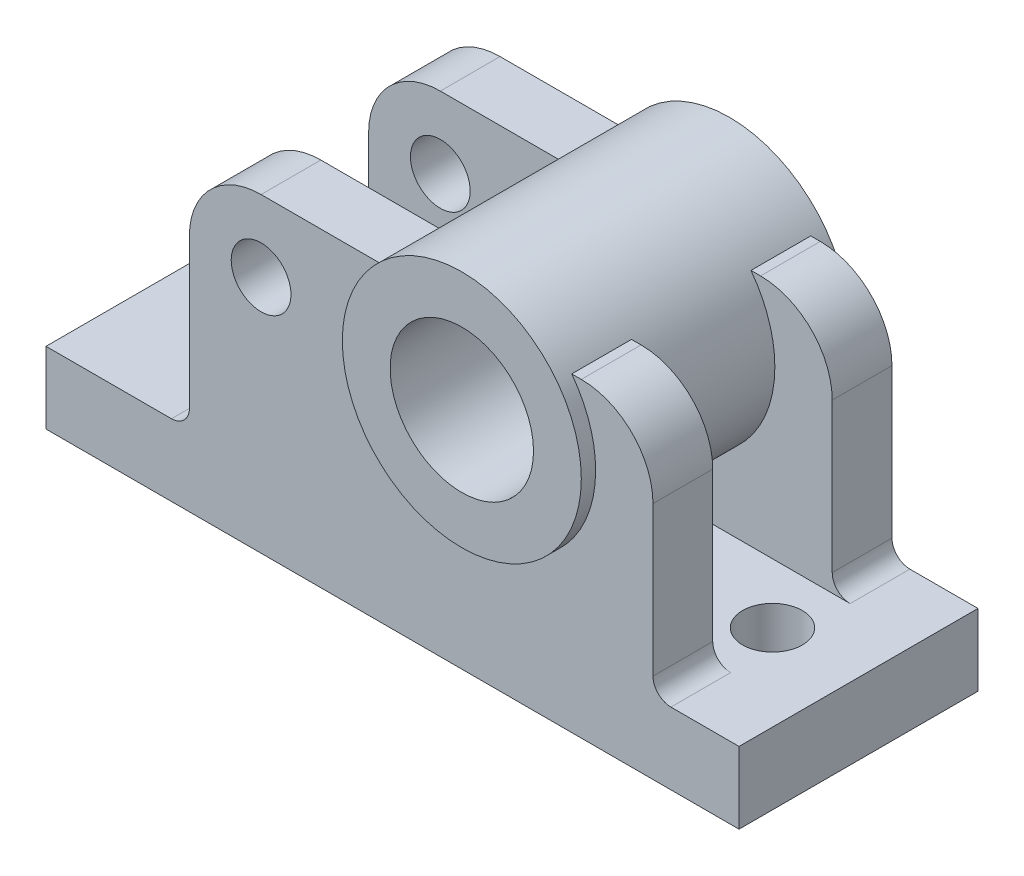
ISO-10303-21;
HEADER;
FILE_DESCRIPTION(('STEP AP214'),'2;1');
FILE_NAME('part.step','',(''),(''),'','','');
FILE_SCHEMA(('AUTOMOTIVE_DESIGN { 1 0 10303 214 1 1 1 1 }'));
ENDSEC;
DATA;
#1=APPLICATION_CONTEXT('core data for automotive mechanical design processes');
#2=APPLICATION_PROTOCOL_DEFINITION('international standard','automotive_design',2000,#1);
#3=PRODUCT_CONTEXT('',#1,'mechanical');
#4=PRODUCT('Part','Part','',(#3));
#5=PRODUCT_RELATED_PRODUCT_CATEGORY('part','',(#4));
#6=PRODUCT_DEFINITION_FORMATION('','',#4);
#7=PRODUCT_DEFINITION_CONTEXT('part definition',#1,'design');
#8=PRODUCT_DEFINITION('design','',#6,#7);
#9=PRODUCT_DEFINITION_SHAPE('','',#8);
#10=(LENGTH_UNIT() NAMED_UNIT(*) SI_UNIT(.MILLI.,.METRE.));
#11=(NAMED_UNIT(*) PLANE_ANGLE_UNIT() SI_UNIT($,.RADIAN.));
#12=(NAMED_UNIT(*) SI_UNIT($,.STERADIAN.) SOLID_ANGLE_UNIT());
#13=UNCERTAINTY_MEASURE_WITH_UNIT(LENGTH_MEASURE(1.E-05),#10,'distance_accuracy_value','');
#14=(GEOMETRIC_REPRESENTATION_CONTEXT(3) GLOBAL_UNCERTAINTY_ASSIGNED_CONTEXT((#13)) GLOBAL_UNIT_ASSIGNED_CONTEXT((#10,
#11,#12)) REPRESENTATION_CONTEXT('',''));
#15=CARTESIAN_POINT('',(0.,0.,0.));
#16=DIRECTION('',(0.,0.,1.));
#17=DIRECTION('',(1.,0.,0.));
#18=AXIS2_PLACEMENT_3D('',#15,#16,#17);
#19=CARTESIAN_POINT('',(110.,30.,50.));
#20=DIRECTION('',(0.,-1.,0.));
#21=DIRECTION('',(0.,0.,-1.));
#22=AXIS2_PLACEMENT_3D('',#19,#20,#21);
#23=PLANE('',#22);
#24=CARTESIAN_POINT('',(-144.,30.,0.));
#25=DIRECTION('',(0.,-1.,0.));
#26=DIRECTION('',(0.,0.,-1.));
#27=AXIS2_PLACEMENT_3D('',#24,#25,#26);
#28=CIRCLE('',#27,12.5);
#29=CARTESIAN_POINT('',(-144.,30.,-12.5));
#30=VERTEX_POINT('',#29);
#31=EDGE_CURVE('E249',#30,#30,#28,.T.);
#32=ORIENTED_EDGE('',*,*,#31,.T.);
#33=EDGE_LOOP('',(#32));
#34=FACE_BOUND('',#33,.T.);
#35=CARTESIAN_POINT('',(74.,30.,0.));
#36=DIRECTION('',(0.,-1.,0.));
#37=DIRECTION('',(0.,0.,-1.));
#38=AXIS2_PLACEMENT_3D('',#35,#36,#37);
#39=CIRCLE('',#38,12.5);
#40=CARTESIAN_POINT('',(74.,30.,-12.5));
#41=VERTEX_POINT('',#40);
#42=EDGE_CURVE('E244',#41,#41,#39,.T.);
#43=ORIENTED_EDGE('',*,*,#42,.T.);
#44=EDGE_LOOP('',(#43));
#45=FACE_BOUND('',#44,.T.);
#46=DIRECTION('',(-1.,0.,0.));
#47=VECTOR('',#46,1.);
#48=CARTESIAN_POINT('',(110.,30.,-50.));
#49=LINE('',#48,#47);
#50=CARTESIAN_POINT('',(110.,30.,-50.));
#51=VERTEX_POINT('',#50);
#52=CARTESIAN_POINT('',(81.5,30.,-50.));
#53=VERTEX_POINT('',#52);
#54=EDGE_CURVE('E64',#51,#53,#49,.T.);
#55=ORIENTED_EDGE('',*,*,#54,.T.);
#56=DIRECTION('',(0.,0.,1.));
#57=VECTOR('',#56,1.);
#58=CARTESIAN_POINT('',(81.5,30.,-50.));
#59=LINE('',#58,#57);
#60=CARTESIAN_POINT('',(81.5,30.,-25.));
#61=VERTEX_POINT('',#60);
#62=EDGE_CURVE('E525',#53,#61,#59,.T.);
#63=ORIENTED_EDGE('',*,*,#62,.T.);
#64=DIRECTION('',(-1.,0.,0.));
#65=VECTOR('',#64,1.);
#66=CARTESIAN_POINT('',(110.,30.,-25.));
#67=LINE('',#66,#65);
#68=CARTESIAN_POINT('',(-127.5,30.,-25.));
#69=VERTEX_POINT('',#68);
#70=EDGE_CURVE('E57',#61,#69,#67,.T.);
#71=ORIENTED_EDGE('',*,*,#70,.T.);
#72=DIRECTION('',(0.,0.,1.));
#73=VECTOR('',#72,1.);
#74=CARTESIAN_POINT('',(-127.5,30.,-50.));
#75=LINE('',#74,#73);
#76=CARTESIAN_POINT('',(-127.5,30.,-50.));
#77=VERTEX_POINT('',#76);
#78=EDGE_CURVE('E207',#77,#69,#75,.T.);
#79=ORIENTED_EDGE('',*,*,#78,.F.);
#80=CARTESIAN_POINT('',(-180.,30.,-50.));
#81=VERTEX_POINT('',#80);
#82=EDGE_CURVE('E217',#77,#81,#49,.T.);
#83=ORIENTED_EDGE('',*,*,#82,.T.);
#84=DIRECTION('',(0.,0.,-1.));
#85=VECTOR('',#84,1.);
#86=CARTESIAN_POINT('',(-180.,30.,50.));
#87=LINE('',#86,#85);
#88=CARTESIAN_POINT('',(-180.,30.,50.));
#89=VERTEX_POINT('',#88);
#90=EDGE_CURVE('E236',#89,#81,#87,.T.);
#91=ORIENTED_EDGE('',*,*,#90,.F.);
#92=DIRECTION('',(-1.,0.,0.));
#93=VECTOR('',#92,1.);
#94=CARTESIAN_POINT('',(110.,30.,50.));
#95=LINE('',#94,#93);
#96=CARTESIAN_POINT('',(-127.5,30.,50.));
#97=VERTEX_POINT('',#96);
#98=EDGE_CURVE('E354',#97,#89,#95,.T.);
#99=ORIENTED_EDGE('',*,*,#98,.F.);
#100=DIRECTION('',(0.,0.,1.));
#101=VECTOR('',#100,1.);
#102=CARTESIAN_POINT('',(-127.5,29.9999999999999,25.));
#103=LINE('',#102,#101);
#104=CARTESIAN_POINT('',(-127.5,29.9999999999999,25.));
#105=VERTEX_POINT('',#104);
#106=EDGE_CURVE('E385',#105,#97,#103,.T.);
#107=ORIENTED_EDGE('',*,*,#106,.F.);
#108=DIRECTION('',(1.,0.,0.));
#109=VECTOR('',#108,1.);
#110=CARTESIAN_POINT('',(-120.,29.9999999999999,25.));
#111=LINE('',#110,#109);
#112=CARTESIAN_POINT('',(81.5,30.,25.));
#113=VERTEX_POINT('',#112);
#114=EDGE_CURVE('E242',#105,#113,#111,.T.);
#115=ORIENTED_EDGE('',*,*,#114,.T.);
#116=DIRECTION('',(0.,0.,1.));
#117=VECTOR('',#116,1.);
#118=CARTESIAN_POINT('',(81.5,29.9999999999999,25.));
#119=LINE('',#118,#117);
#120=CARTESIAN_POINT('',(81.5,30.,50.));
#121=VERTEX_POINT('',#120);
#122=EDGE_CURVE('E540',#113,#121,#119,.T.);
#123=ORIENTED_EDGE('',*,*,#122,.T.);
#124=CARTESIAN_POINT('',(110.,30.,50.));
#125=VERTEX_POINT('',#124);
#126=EDGE_CURVE('E358',#125,#121,#95,.T.);
#127=ORIENTED_EDGE('',*,*,#126,.F.);
#128=DIRECTION('',(0.,0.,-1.));
#129=VECTOR('',#128,1.);
#130=CARTESIAN_POINT('',(110.,30.,50.));
#131=LINE('',#130,#129);
#132=EDGE_CURVE('E237',#125,#51,#131,.T.);
#133=ORIENTED_EDGE('',*,*,#132,.T.);
#134=EDGE_LOOP('',(#55,#63,#71,#79,#83,#91,#99,#107,#115,#123,#127,#133));
#135=FACE_BOUND('',#134,.T.);
#136=ADVANCED_FACE('F41',(#34,#45,#135),#23,.F.);
#137=CARTESIAN_POINT('',(-120.,130.,-50.));
#138=DIRECTION('',(-1.,0.,0.));
#139=DIRECTION('',(0.,0.,1.));
#140=AXIS2_PLACEMENT_3D('',#137,#138,#139);
#141=PLANE('',#140);
#142=DIRECTION('',(0.,-1.,0.));
#143=VECTOR('',#142,1.);
#144=CARTESIAN_POINT('',(-120.,130.,-50.));
#145=LINE('',#144,#143);
#146=CARTESIAN_POINT('',(-120.,99.9999999999999,-50.));
#147=VERTEX_POINT('',#146);
#148=CARTESIAN_POINT('',(-120.,37.5,-50.));
#149=VERTEX_POINT('',#148);
#150=EDGE_CURVE('E319',#147,#149,#145,.T.);
#151=ORIENTED_EDGE('',*,*,#150,.T.);
#152=DIRECTION('',(0.,0.,1.));
#153=VECTOR('',#152,1.);
#154=CARTESIAN_POINT('',(-120.,37.5,-50.));
#155=LINE('',#154,#153);
#156=CARTESIAN_POINT('',(-120.,37.5,-25.));
#157=VERTEX_POINT('',#156);
#158=EDGE_CURVE('E206',#149,#157,#155,.T.);
#159=ORIENTED_EDGE('',*,*,#158,.T.);
#160=DIRECTION('',(0.,-1.,0.));
#161=VECTOR('',#160,1.);
#162=CARTESIAN_POINT('',(-120.,130.,-25.));
#163=LINE('',#162,#161);
#164=CARTESIAN_POINT('',(-120.,99.9999999999999,-25.));
#165=VERTEX_POINT('',#164);
#166=EDGE_CURVE('E340',#165,#157,#163,.T.);
#167=ORIENTED_EDGE('',*,*,#166,.F.);
#168=DIRECTION('',(0.,0.,1.));
#169=VECTOR('',#168,1.);
#170=CARTESIAN_POINT('',(-120.,99.9999999999999,-80.));
#171=LINE('',#170,#169);
#172=EDGE_CURVE('E413',#147,#165,#171,.T.);
#173=ORIENTED_EDGE('',*,*,#172,.F.);
#174=EDGE_LOOP('',(#151,#159,#167,#173));
#175=FACE_BOUND('',#174,.T.);
#176=ADVANCED_FACE('F450',(#175),#141,.T.);
#177=CARTESIAN_POINT('',(-120.,130.,50.));
#178=DIRECTION('',(1.,0.,0.));
#179=DIRECTION('',(0.,0.,-1.));
#180=AXIS2_PLACEMENT_3D('',#177,#178,#179);
#181=PLANE('',#180);
#182=DIRECTION('',(0.,0.,1.));
#183=VECTOR('',#182,1.);
#184=CARTESIAN_POINT('',(-120.,37.5,25.));
#185=LINE('',#184,#183);
#186=CARTESIAN_POINT('',(-120.,37.5,25.));
#187=VERTEX_POINT('',#186);
#188=CARTESIAN_POINT('',(-120.,37.5,50.));
#189=VERTEX_POINT('',#188);
#190=EDGE_CURVE('E387',#187,#189,#185,.T.);
#191=ORIENTED_EDGE('',*,*,#190,.T.);
#192=DIRECTION('',(0.,-1.,0.));
#193=VECTOR('',#192,1.);
#194=CARTESIAN_POINT('',(-120.,130.,50.));
#195=LINE('',#194,#193);
#196=CARTESIAN_POINT('',(-120.,99.9999999999999,50.));
#197=VERTEX_POINT('',#196);
#198=EDGE_CURVE('E264',#197,#189,#195,.T.);
#199=ORIENTED_EDGE('',*,*,#198,.F.);
#200=CARTESIAN_POINT('',(-120.,99.9999999999999,25.));
#201=VERTEX_POINT('',#200);
#202=EDGE_CURVE('E415',#201,#197,#171,.T.);
#203=ORIENTED_EDGE('',*,*,#202,.F.);
#204=DIRECTION('',(0.,-1.,0.));
#205=VECTOR('',#204,1.);
#206=CARTESIAN_POINT('',(-120.,130.,25.));
#207=LINE('',#206,#205);
#208=EDGE_CURVE('E266',#201,#187,#207,.T.);
#209=ORIENTED_EDGE('',*,*,#208,.T.);
#210=EDGE_LOOP('',(#191,#199,#203,#209));
#211=FACE_BOUND('',#210,.T.);
#212=ADVANCED_FACE('F453',(#211),#181,.F.);
#213=CARTESIAN_POINT('',(-120.,130.,25.));
#214=DIRECTION('',(0.,0.,1.));
#215=DIRECTION('',(1.,0.,0.));
#216=AXIS2_PLACEMENT_3D('',#213,#214,#215);
#217=PLANE('',#216);
#218=CARTESIAN_POINT('',(-90.,99.9999999999999,25.));
#219=DIRECTION('',(0.,0.,1.));
#220=DIRECTION('',(1.,0.,0.));
#221=AXIS2_PLACEMENT_3D('',#218,#219,#220);
#222=CIRCLE('',#221,12.5);
#223=CARTESIAN_POINT('',(-77.5,99.9999999999999,25.));
#224=VERTEX_POINT('',#223);
#225=EDGE_CURVE('E330',#224,#224,#222,.T.);
#226=ORIENTED_EDGE('',*,*,#225,.T.);
#227=EDGE_LOOP('',(#226));
#228=FACE_BOUND('',#227,.T.);
#229=CARTESIAN_POINT('',(44.,100.,25.));
#230=DIRECTION('',(0.,0.,1.));
#231=DIRECTION('',(1.,0.,0.));
#232=AXIS2_PLACEMENT_3D('',#229,#230,#231);
#233=CIRCLE('',#232,30.);
#234=CARTESIAN_POINT('',(74.,100.,25.));
#235=VERTEX_POINT('',#234);
#236=CARTESIAN_POINT('',(43.9999999999999,130.,25.));
#237=VERTEX_POINT('',#236);
#238=EDGE_CURVE('E409',#235,#237,#233,.T.);
#239=ORIENTED_EDGE('',*,*,#238,.F.);
#240=DIRECTION('',(0.,-1.,0.));
#241=VECTOR('',#240,1.);
#242=CARTESIAN_POINT('',(74.,130.,25.));
#243=LINE('',#242,#241);
#244=CARTESIAN_POINT('',(74.,37.5,25.));
#245=VERTEX_POINT('',#244);
#246=EDGE_CURVE('E268',#235,#245,#243,.T.);
#247=ORIENTED_EDGE('',*,*,#246,.T.);
#248=CARTESIAN_POINT('',(81.5,37.5,25.));
#249=DIRECTION('',(0.,0.,-1.));
#250=DIRECTION('',(1.,0.,0.));
#251=AXIS2_PLACEMENT_3D('',#248,#249,#250);
#252=CIRCLE('',#251,7.50000000000001);
#253=EDGE_CURVE('E535',#113,#245,#252,.T.);
#254=ORIENTED_EDGE('',*,*,#253,.F.);
#255=ORIENTED_EDGE('',*,*,#114,.F.);
#256=CARTESIAN_POINT('',(-127.5,37.5,25.));
#257=DIRECTION('',(0.,0.,-1.));
#258=DIRECTION('',(1.,0.,0.));
#259=AXIS2_PLACEMENT_3D('',#256,#257,#258);
#260=CIRCLE('',#259,7.50000000000001);
#261=EDGE_CURVE('E390',#187,#105,#260,.T.);
#262=ORIENTED_EDGE('',*,*,#261,.F.);
#263=ORIENTED_EDGE('',*,*,#208,.F.);
#264=CARTESIAN_POINT('',(-90.,99.9999999999999,25.));
#265=DIRECTION('',(0.,0.,1.));
#266=DIRECTION('',(1.,0.,0.));
#267=AXIS2_PLACEMENT_3D('',#264,#265,#266);
#268=CIRCLE('',#267,30.0000000000001);
#269=CARTESIAN_POINT('',(-90.,130.,25.));
#270=VERTEX_POINT('',#269);
#271=EDGE_CURVE('E305',#201,#270,#268,.F.);
#272=ORIENTED_EDGE('',*,*,#271,.T.);
#273=DIRECTION('',(-1.,0.,0.));
#274=VECTOR('',#273,1.);
#275=CARTESIAN_POINT('',(-120.,130.,25.));
#276=LINE('',#275,#274);
#277=CARTESIAN_POINT('',(-40.,130.,25.));
#278=VERTEX_POINT('',#277);
#279=EDGE_CURVE('E259',#278,#270,#276,.T.);
#280=ORIENTED_EDGE('',*,*,#279,.F.);
#281=CARTESIAN_POINT('',(0.,99.9999999999999,25.));
#282=DIRECTION('',(0.,0.,1.));
#283=DIRECTION('',(1.,0.,0.));
#284=AXIS2_PLACEMENT_3D('',#281,#282,#283);
#285=CIRCLE('',#284,50.);
#286=CARTESIAN_POINT('',(40.,130.,25.));
#287=VERTEX_POINT('',#286);
#288=EDGE_CURVE('E278',#278,#287,#285,.T.);
#289=ORIENTED_EDGE('',*,*,#288,.T.);
#290=EDGE_CURVE('E258',#237,#287,#276,.T.);
#291=ORIENTED_EDGE('',*,*,#290,.F.);
#292=EDGE_LOOP('',(#239,#247,#254,#255,#262,#263,#272,#280,#289,#291));
#293=FACE_BOUND('',#292,.T.);
#294=ADVANCED_FACE('F426',(#228,#293),#217,.F.);
#295=CARTESIAN_POINT('',(0.,130.,0.));
#296=DIRECTION('',(0.,-1.,0.));
#297=DIRECTION('',(0.,0.,-1.));
#298=AXIS2_PLACEMENT_3D('',#295,#296,#297);
#299=PLANE('',#298);
#300=DIRECTION('',(0.,0.,1.));
#301=VECTOR('',#300,1.);
#302=CARTESIAN_POINT('',(43.9999999999999,130.,-60.));
#303=LINE('',#302,#301);
#304=CARTESIAN_POINT('',(43.9999999999999,130.,50.));
#305=VERTEX_POINT('',#304);
#306=EDGE_CURVE('E397',#237,#305,#303,.T.);
#307=ORIENTED_EDGE('',*,*,#306,.F.);
#308=ORIENTED_EDGE('',*,*,#290,.T.);
#309=DIRECTION('',(0.,0.,-1.));
#310=VECTOR('',#309,1.);
#311=CARTESIAN_POINT('',(40.,130.,56.));
#312=LINE('',#311,#310);
#313=CARTESIAN_POINT('',(40.,130.,50.));
#314=VERTEX_POINT('',#313);
#315=EDGE_CURVE('E274',#287,#314,#312,.F.);
#316=ORIENTED_EDGE('',*,*,#315,.T.);
#317=DIRECTION('',(1.,0.,0.));
#318=VECTOR('',#317,1.);
#319=CARTESIAN_POINT('',(74.,130.,50.));
#320=LINE('',#319,#318);
#321=EDGE_CURVE('E256',#314,#305,#320,.T.);
#322=ORIENTED_EDGE('',*,*,#321,.T.);
#323=EDGE_LOOP('',(#307,#308,#316,#322));
#324=FACE_BOUND('',#323,.T.);
#325=ADVANCED_FACE('F466',(#324),#299,.F.);
#326=CARTESIAN_POINT('',(74.,130.,50.));
#327=DIRECTION('',(0.,0.,-1.));
#328=DIRECTION('',(-1.,0.,0.));
#329=AXIS2_PLACEMENT_3D('',#326,#327,#328);
#330=PLANE('',#329);
#331=ORIENTED_EDGE('',*,*,#126,.T.);
#332=CARTESIAN_POINT('',(81.5,37.5,50.));
#333=DIRECTION('',(0.,0.,-1.));
#334=DIRECTION('',(1.,0.,0.));
#335=AXIS2_PLACEMENT_3D('',#332,#333,#334);
#336=CIRCLE('',#335,7.50000000000001);
#337=CARTESIAN_POINT('',(74.,37.5,50.));
#338=VERTEX_POINT('',#337);
#339=EDGE_CURVE('E526',#121,#338,#336,.T.);
#340=ORIENTED_EDGE('',*,*,#339,.T.);
#341=DIRECTION('',(0.,-1.,0.));
#342=VECTOR('',#341,1.);
#343=CARTESIAN_POINT('',(74.,130.,50.));
#344=LINE('',#343,#342);
#345=CARTESIAN_POINT('',(74.,100.,50.));
#346=VERTEX_POINT('',#345);
#347=EDGE_CURVE('E275',#346,#338,#344,.T.);
#348=ORIENTED_EDGE('',*,*,#347,.F.);
#349=CARTESIAN_POINT('',(44.,100.,50.));
#350=DIRECTION('',(0.,0.,1.));
#351=DIRECTION('',(1.,0.,0.));
#352=AXIS2_PLACEMENT_3D('',#349,#350,#351);
#353=CIRCLE('',#352,30.);
#354=EDGE_CURVE('E388',#346,#305,#353,.T.);
#355=ORIENTED_EDGE('',*,*,#354,.T.);
#356=ORIENTED_EDGE('',*,*,#321,.F.);
#357=CARTESIAN_POINT('',(0.,99.9999999999999,50.));
#358=DIRECTION('',(0.,0.,-1.));
#359=DIRECTION('',(-1.,0.,0.));
#360=AXIS2_PLACEMENT_3D('',#357,#358,#359);
#361=CIRCLE('',#360,50.);
#362=CARTESIAN_POINT('',(-40.,130.,50.));
#363=VERTEX_POINT('',#362);
#364=EDGE_CURVE('E285',#314,#363,#361,.T.);
#365=ORIENTED_EDGE('',*,*,#364,.T.);
#366=CARTESIAN_POINT('',(-90.,130.,50.));
#367=VERTEX_POINT('',#366);
#368=EDGE_CURVE('E257',#367,#363,#320,.T.);
#369=ORIENTED_EDGE('',*,*,#368,.F.);
#370=CARTESIAN_POINT('',(-90.,99.9999999999999,50.));
#371=DIRECTION('',(0.,0.,-1.));
#372=DIRECTION('',(1.,0.,0.));
#373=AXIS2_PLACEMENT_3D('',#370,#371,#372);
#374=CIRCLE('',#373,30.0000000000001);
#375=EDGE_CURVE('E408',#197,#367,#374,.T.);
#376=ORIENTED_EDGE('',*,*,#375,.F.);
#377=ORIENTED_EDGE('',*,*,#198,.T.);
#378=CARTESIAN_POINT('',(-127.5,37.5,50.));
#379=DIRECTION('',(0.,0.,-1.));
#380=DIRECTION('',(1.,0.,0.));
#381=AXIS2_PLACEMENT_3D('',#378,#379,#380);
#382=CIRCLE('',#381,7.50000000000001);
#383=EDGE_CURVE('E220',#189,#97,#382,.T.);
#384=ORIENTED_EDGE('',*,*,#383,.T.);
#385=ORIENTED_EDGE('',*,*,#98,.T.);
#386=DIRECTION('',(0.,-1.,0.));
#387=VECTOR('',#386,1.);
#388=CARTESIAN_POINT('',(-180.,0.,50.));
#389=LINE('',#388,#387);
#390=CARTESIAN_POINT('',(-180.,0.,50.));
#391=VERTEX_POINT('',#390);
#392=EDGE_CURVE('E240',#89,#391,#389,.T.);
#393=ORIENTED_EDGE('',*,*,#392,.T.);
#394=DIRECTION('',(1.,0.,0.));
#395=VECTOR('',#394,1.);
#396=CARTESIAN_POINT('',(74.,0.,50.));
#397=LINE('',#396,#395);
#398=CARTESIAN_POINT('',(110.,0.,50.));
#399=VERTEX_POINT('',#398);
#400=EDGE_CURVE('E253',#391,#399,#397,.T.);
#401=ORIENTED_EDGE('',*,*,#400,.T.);
#402=DIRECTION('',(0.,1.,0.));
#403=VECTOR('',#402,1.);
#404=CARTESIAN_POINT('',(110.,0.,50.));
#405=LINE('',#404,#403);
#406=EDGE_CURVE('E235',#399,#125,#405,.T.);
#407=ORIENTED_EDGE('',*,*,#406,.T.);
#408=EDGE_LOOP('',(#331,#340,#348,#355,#356,#365,#369,#376,#377,#384,#385,#393,#401,#407));
#409=FACE_BOUND('',#408,.T.);
#410=CARTESIAN_POINT('',(-90.,99.9999999999999,50.));
#411=DIRECTION('',(0.,0.,-1.));
#412=DIRECTION('',(-1.,0.,0.));
#413=AXIS2_PLACEMENT_3D('',#410,#411,#412);
#414=CIRCLE('',#413,12.5);
#415=CARTESIAN_POINT('',(-102.5,99.9999999999999,50.));
#416=VERTEX_POINT('',#415);
#417=EDGE_CURVE('E422',#416,#416,#414,.T.);
#418=ORIENTED_EDGE('',*,*,#417,.T.);
#419=EDGE_LOOP('',(#418));
#420=FACE_BOUND('',#419,.T.);
#421=ADVANCED_FACE('F375',(#409,#420),#330,.F.);
#422=CARTESIAN_POINT('',(0.,0.,-50.));
#423=DIRECTION('',(0.,0.,1.));
#424=DIRECTION('',(1.,0.,0.));
#425=AXIS2_PLACEMENT_3D('',#422,#423,#424);
#426=PLANE('',#425);
#427=CARTESIAN_POINT('',(-90.,99.9999999999999,-50.));
#428=DIRECTION('',(0.,0.,1.));
#429=DIRECTION('',(1.,0.,0.));
#430=AXIS2_PLACEMENT_3D('',#427,#428,#429);
#431=CIRCLE('',#430,12.5);
#432=CARTESIAN_POINT('',(-77.5,99.9999999999999,-50.));
#433=VERTEX_POINT('',#432);
#434=EDGE_CURVE('E301',#433,#433,#431,.T.);
#435=ORIENTED_EDGE('',*,*,#434,.T.);
#436=EDGE_LOOP('',(#435));
#437=FACE_BOUND('',#436,.T.);
#438=CARTESIAN_POINT('',(44.,100.,-50.));
#439=DIRECTION('',(0.,0.,1.));
#440=DIRECTION('',(1.,0.,0.));
#441=AXIS2_PLACEMENT_3D('',#438,#439,#440);
#442=CIRCLE('',#441,30.);
#443=CARTESIAN_POINT('',(74.,100.,-50.));
#444=VERTEX_POINT('',#443);
#445=CARTESIAN_POINT('',(44.,130.,-50.));
#446=VERTEX_POINT('',#445);
#447=EDGE_CURVE('E407',#444,#446,#442,.T.);
#448=ORIENTED_EDGE('',*,*,#447,.F.);
#449=DIRECTION('',(0.,-1.,0.));
#450=VECTOR('',#449,1.);
#451=CARTESIAN_POINT('',(74.,130.,-50.));
#452=LINE('',#451,#450);
#453=CARTESIAN_POINT('',(74.,37.5,-50.));
#454=VERTEX_POINT('',#453);
#455=EDGE_CURVE('E335',#444,#454,#452,.T.);
#456=ORIENTED_EDGE('',*,*,#455,.T.);
#457=CARTESIAN_POINT('',(81.5,37.5,-50.));
#458=DIRECTION('',(0.,0.,1.));
#459=DIRECTION('',(1.,0.,0.));
#460=AXIS2_PLACEMENT_3D('',#457,#458,#459);
#461=CIRCLE('',#460,7.5);
#462=EDGE_CURVE('E521',#454,#53,#461,.T.);
#463=ORIENTED_EDGE('',*,*,#462,.T.);
#464=ORIENTED_EDGE('',*,*,#54,.F.);
#465=DIRECTION('',(0.,1.,0.));
#466=VECTOR('',#465,1.);
#467=CARTESIAN_POINT('',(110.,0.,-50.));
#468=LINE('',#467,#466);
#469=CARTESIAN_POINT('',(110.,0.,-50.));
#470=VERTEX_POINT('',#469);
#471=EDGE_CURVE('E224',#470,#51,#468,.T.);
#472=ORIENTED_EDGE('',*,*,#471,.F.);
#473=DIRECTION('',(1.,0.,0.));
#474=VECTOR('',#473,1.);
#475=CARTESIAN_POINT('',(-180.,0.,-50.));
#476=LINE('',#475,#474);
#477=CARTESIAN_POINT('',(-180.,0.,-50.));
#478=VERTEX_POINT('',#477);
#479=EDGE_CURVE('E227',#478,#470,#476,.T.);
#480=ORIENTED_EDGE('',*,*,#479,.F.);
#481=DIRECTION('',(0.,-1.,0.));
#482=VECTOR('',#481,1.);
#483=CARTESIAN_POINT('',(-180.,0.,-50.));
#484=LINE('',#483,#482);
#485=EDGE_CURVE('E223',#81,#478,#484,.T.);
#486=ORIENTED_EDGE('',*,*,#485,.F.);
#487=ORIENTED_EDGE('',*,*,#82,.F.);
#488=CARTESIAN_POINT('',(-127.5,37.5,-50.));
#489=DIRECTION('',(0.,0.,1.));
#490=DIRECTION('',(1.,0.,0.));
#491=AXIS2_PLACEMENT_3D('',#488,#489,#490);
#492=CIRCLE('',#491,7.5);
#493=EDGE_CURVE('E202',#77,#149,#492,.T.);
#494=ORIENTED_EDGE('',*,*,#493,.T.);
#495=ORIENTED_EDGE('',*,*,#150,.F.);
#496=CARTESIAN_POINT('',(-90.,99.9999999999999,-50.));
#497=DIRECTION('',(0.,0.,1.));
#498=DIRECTION('',(1.,0.,0.));
#499=AXIS2_PLACEMENT_3D('',#496,#497,#498);
#500=CIRCLE('',#499,30.0000000000001);
#501=CARTESIAN_POINT('',(-90.,130.,-50.));
#502=VERTEX_POINT('',#501);
#503=EDGE_CURVE('E310',#147,#502,#500,.F.);
#504=ORIENTED_EDGE('',*,*,#503,.T.);
#505=DIRECTION('',(1.,0.,0.));
#506=VECTOR('',#505,1.);
#507=CARTESIAN_POINT('',(74.,130.,-50.));
#508=LINE('',#507,#506);
#509=CARTESIAN_POINT('',(-40.,130.,-50.));
#510=VERTEX_POINT('',#509);
#511=EDGE_CURVE('E317',#502,#510,#508,.T.);
#512=ORIENTED_EDGE('',*,*,#511,.T.);
#513=CARTESIAN_POINT('',(0.,99.9999999999999,-50.));
#514=DIRECTION('',(0.,0.,-1.));
#515=DIRECTION('',(-1.,0.,0.));
#516=AXIS2_PLACEMENT_3D('',#513,#514,#515);
#517=CIRCLE('',#516,50.);
#518=CARTESIAN_POINT('',(40.,130.,-50.));
#519=VERTEX_POINT('',#518);
#520=EDGE_CURVE('E341',#519,#510,#517,.T.);
#521=ORIENTED_EDGE('',*,*,#520,.F.);
#522=EDGE_CURVE('E324',#519,#446,#508,.T.);
#523=ORIENTED_EDGE('',*,*,#522,.T.);
#524=EDGE_LOOP('',(#448,#456,#463,#464,#472,#480,#486,#487,#494,#495,#504,#512,#521,#523));
#525=FACE_BOUND('',#524,.T.);
#526=ADVANCED_FACE('F225',(#437,#525),#426,.F.);
#527=CARTESIAN_POINT('',(74.,130.,-25.));
#528=DIRECTION('',(1.,0.,0.));
#529=DIRECTION('',(0.,0.,-1.));
#530=AXIS2_PLACEMENT_3D('',#527,#528,#529);
#531=PLANE('',#530);
#532=DIRECTION('',(0.,0.,1.));
#533=VECTOR('',#532,1.);
#534=CARTESIAN_POINT('',(74.,37.5,-50.));
#535=LINE('',#534,#533);
#536=CARTESIAN_POINT('',(74.,37.5,-25.));
#537=VERTEX_POINT('',#536);
#538=EDGE_CURVE('E518',#454,#537,#535,.T.);
#539=ORIENTED_EDGE('',*,*,#538,.F.);
#540=ORIENTED_EDGE('',*,*,#455,.F.);
#541=DIRECTION('',(0.,0.,1.));
#542=VECTOR('',#541,1.);
#543=CARTESIAN_POINT('',(74.,100.,-60.));
#544=LINE('',#543,#542);
#545=CARTESIAN_POINT('',(74.,100.,-25.));
#546=VERTEX_POINT('',#545);
#547=EDGE_CURVE('E402',#444,#546,#544,.T.);
#548=ORIENTED_EDGE('',*,*,#547,.T.);
#549=DIRECTION('',(0.,-1.,0.));
#550=VECTOR('',#549,1.);
#551=CARTESIAN_POINT('',(74.,130.,-25.));
#552=LINE('',#551,#550);
#553=EDGE_CURVE('E334',#546,#537,#552,.T.);
#554=ORIENTED_EDGE('',*,*,#553,.T.);
#555=EDGE_LOOP('',(#539,#540,#548,#554));
#556=FACE_BOUND('',#555,.T.);
#557=ADVANCED_FACE('F519',(#556),#531,.T.);
#558=CARTESIAN_POINT('',(-120.,130.,-25.));
#559=DIRECTION('',(0.,0.,1.));
#560=DIRECTION('',(1.,0.,0.));
#561=AXIS2_PLACEMENT_3D('',#558,#559,#560);
#562=PLANE('',#561);
#563=CARTESIAN_POINT('',(-90.,99.9999999999999,-25.));
#564=DIRECTION('',(0.,0.,1.));
#565=DIRECTION('',(1.,0.,0.));
#566=AXIS2_PLACEMENT_3D('',#563,#564,#565);
#567=CIRCLE('',#566,12.5);
#568=CARTESIAN_POINT('',(-77.5,99.9999999999999,-25.));
#569=VERTEX_POINT('',#568);
#570=EDGE_CURVE('E299',#569,#569,#567,.T.);
#571=ORIENTED_EDGE('',*,*,#570,.F.);
#572=EDGE_LOOP('',(#571));
#573=FACE_BOUND('',#572,.T.);
#574=ORIENTED_EDGE('',*,*,#553,.F.);
#575=CARTESIAN_POINT('',(44.,100.,-25.));
#576=DIRECTION('',(0.,0.,1.));
#577=DIRECTION('',(1.,0.,0.));
#578=AXIS2_PLACEMENT_3D('',#575,#576,#577);
#579=CIRCLE('',#578,30.);
#580=CARTESIAN_POINT('',(43.9999999999999,130.,-25.));
#581=VERTEX_POINT('',#580);
#582=EDGE_CURVE('E399',#546,#581,#579,.T.);
#583=ORIENTED_EDGE('',*,*,#582,.T.);
#584=DIRECTION('',(-1.,0.,0.));
#585=VECTOR('',#584,1.);
#586=CARTESIAN_POINT('',(-120.,130.,-25.));
#587=LINE('',#586,#585);
#588=CARTESIAN_POINT('',(40.,130.,-25.));
#589=VERTEX_POINT('',#588);
#590=EDGE_CURVE('E323',#581,#589,#587,.T.);
#591=ORIENTED_EDGE('',*,*,#590,.T.);
#592=CARTESIAN_POINT('',(0.,99.9999999999999,-25.));
#593=DIRECTION('',(0.,0.,1.));
#594=DIRECTION('',(1.,0.,0.));
#595=AXIS2_PLACEMENT_3D('',#592,#593,#594);
#596=CIRCLE('',#595,50.);
#597=CARTESIAN_POINT('',(-40.,130.,-25.));
#598=VERTEX_POINT('',#597);
#599=EDGE_CURVE('E342',#598,#589,#596,.T.);
#600=ORIENTED_EDGE('',*,*,#599,.F.);
#601=CARTESIAN_POINT('',(-90.,130.,-25.));
#602=VERTEX_POINT('',#601);
#603=EDGE_CURVE('E325',#598,#602,#587,.T.);
#604=ORIENTED_EDGE('',*,*,#603,.T.);
#605=CARTESIAN_POINT('',(-90.,99.9999999999999,-25.));
#606=DIRECTION('',(0.,0.,1.));
#607=DIRECTION('',(1.,0.,0.));
#608=AXIS2_PLACEMENT_3D('',#605,#606,#607);
#609=CIRCLE('',#608,30.0000000000001);
#610=EDGE_CURVE('E309',#165,#602,#609,.F.);
#611=ORIENTED_EDGE('',*,*,#610,.F.);
#612=ORIENTED_EDGE('',*,*,#166,.T.);
#613=CARTESIAN_POINT('',(-127.5,37.5,-25.));
#614=DIRECTION('',(0.,0.,1.));
#615=DIRECTION('',(1.,0.,0.));
#616=AXIS2_PLACEMENT_3D('',#613,#614,#615);
#617=CIRCLE('',#616,7.5);
#618=EDGE_CURVE('E214',#69,#157,#617,.T.);
#619=ORIENTED_EDGE('',*,*,#618,.F.);
#620=ORIENTED_EDGE('',*,*,#70,.F.);
#621=CARTESIAN_POINT('',(81.5,37.5,-25.));
#622=DIRECTION('',(0.,0.,1.));
#623=DIRECTION('',(1.,0.,0.));
#624=AXIS2_PLACEMENT_3D('',#621,#622,#623);
#625=CIRCLE('',#624,7.5);
#626=EDGE_CURVE('E527',#537,#61,#625,.T.);
#627=ORIENTED_EDGE('',*,*,#626,.F.);
#628=EDGE_LOOP('',(#574,#583,#591,#600,#604,#611,#612,#619,#620,#627));
#629=FACE_BOUND('',#628,.T.);
#630=ADVANCED_FACE('F507',(#573,#629),#562,.T.);
#631=CARTESIAN_POINT('',(0.,130.,0.));
#632=DIRECTION('',(0.,-1.,0.));
#633=DIRECTION('',(0.,0.,1.));
#634=AXIS2_PLACEMENT_3D('',#631,#632,#633);
#635=PLANE('',#634);
#636=DIRECTION('',(0.,0.,1.));
#637=VECTOR('',#636,1.);
#638=CARTESIAN_POINT('',(44.,130.,-60.));
#639=LINE('',#638,#637);
#640=EDGE_CURVE('E11',#446,#581,#639,.T.);
#641=ORIENTED_EDGE('',*,*,#640,.F.);
#642=ORIENTED_EDGE('',*,*,#522,.F.);
#643=DIRECTION('',(0.,0.,-1.));
#644=VECTOR('',#643,1.);
#645=CARTESIAN_POINT('',(40.,130.,56.));
#646=LINE('',#645,#644);
#647=EDGE_CURVE('E347',#519,#589,#646,.F.);
#648=ORIENTED_EDGE('',*,*,#647,.T.);
#649=ORIENTED_EDGE('',*,*,#590,.F.);
#650=EDGE_LOOP('',(#641,#642,#648,#649));
#651=FACE_BOUND('',#650,.T.);
#652=ADVANCED_FACE('F467',(#651),#635,.F.);
#653=DIRECTION('',(0.,0.,1.));
#654=VECTOR('',#653,1.);
#655=CARTESIAN_POINT('',(-90.,130.,-80.));
#656=LINE('',#655,#654);
#657=EDGE_CURVE('E414',#270,#367,#656,.T.);
#658=ORIENTED_EDGE('',*,*,#657,.T.);
#659=ORIENTED_EDGE('',*,*,#368,.T.);
#660=DIRECTION('',(0.,0.,-1.));
#661=VECTOR('',#660,1.);
#662=CARTESIAN_POINT('',(-40.,130.,56.));
#663=LINE('',#662,#661);
#664=EDGE_CURVE('E280',#363,#278,#663,.T.);
#665=ORIENTED_EDGE('',*,*,#664,.T.);
#666=ORIENTED_EDGE('',*,*,#279,.T.);
#667=EDGE_LOOP('',(#658,#659,#665,#666));
#668=FACE_BOUND('',#667,.T.);
#669=ADVANCED_FACE('F463',(#668),#299,.F.);
#670=DIRECTION('',(0.,0.,1.));
#671=VECTOR('',#670,1.);
#672=CARTESIAN_POINT('',(-90.,130.,-80.));
#673=LINE('',#672,#671);
#674=EDGE_CURVE('E47',#602,#502,#673,.F.);
#675=ORIENTED_EDGE('',*,*,#674,.F.);
#676=ORIENTED_EDGE('',*,*,#603,.F.);
#677=DIRECTION('',(0.,0.,-1.));
#678=VECTOR('',#677,1.);
#679=CARTESIAN_POINT('',(-40.,130.,56.));
#680=LINE('',#679,#678);
#681=EDGE_CURVE('E248',#598,#510,#680,.T.);
#682=ORIENTED_EDGE('',*,*,#681,.T.);
#683=ORIENTED_EDGE('',*,*,#511,.F.);
#684=EDGE_LOOP('',(#675,#676,#682,#683));
#685=FACE_BOUND('',#684,.T.);
#686=ADVANCED_FACE('F322',(#685),#635,.F.);
#687=CARTESIAN_POINT('',(0.,99.9999999999999,56.));
#688=DIRECTION('',(0.,0.,-1.));
#689=DIRECTION('',(-1.,0.,0.));
#690=AXIS2_PLACEMENT_3D('',#687,#688,#689);
#691=CYLINDRICAL_SURFACE('',#690,50.);
#692=ORIENTED_EDGE('',*,*,#664,.F.);
#693=ORIENTED_EDGE('',*,*,#364,.F.);
#694=ORIENTED_EDGE('',*,*,#315,.F.);
#695=ORIENTED_EDGE('',*,*,#288,.F.);
#696=EDGE_LOOP('',(#692,#693,#694,#695));
#697=FACE_BOUND('',#696,.T.);
#698=CARTESIAN_POINT('',(0.,99.9999999999999,56.));
#699=DIRECTION('',(0.,0.,1.));
#700=DIRECTION('',(1.,0.,0.));
#701=AXIS2_PLACEMENT_3D('',#698,#699,#700);
#702=CIRCLE('',#701,50.);
#703=CARTESIAN_POINT('',(50.,99.9999999999999,56.));
#704=VERTEX_POINT('',#703);
#705=EDGE_CURVE('E291',#704,#704,#702,.T.);
#706=ORIENTED_EDGE('',*,*,#705,.F.);
#707=EDGE_LOOP('',(#706));
#708=FACE_BOUND('',#707,.T.);
#709=CARTESIAN_POINT('',(0.,99.9999999999999,-56.));
#710=DIRECTION('',(0.,0.,1.));
#711=DIRECTION('',(1.,0.,0.));
#712=AXIS2_PLACEMENT_3D('',#709,#710,#711);
#713=CIRCLE('',#712,50.);
#714=CARTESIAN_POINT('',(50.,99.9999999999999,-56.));
#715=VERTEX_POINT('',#714);
#716=EDGE_CURVE('E289',#715,#715,#713,.T.);
#717=ORIENTED_EDGE('',*,*,#716,.T.);
#718=EDGE_LOOP('',(#717));
#719=FACE_BOUND('',#718,.T.);
#720=ORIENTED_EDGE('',*,*,#681,.F.);
#721=ORIENTED_EDGE('',*,*,#599,.T.);
#722=ORIENTED_EDGE('',*,*,#647,.F.);
#723=ORIENTED_EDGE('',*,*,#520,.T.);
#724=EDGE_LOOP('',(#720,#721,#722,#723));
#725=FACE_BOUND('',#724,.T.);
#726=ADVANCED_FACE('F43',(#697,#708,#719,#725),#691,.T.);
#727=CARTESIAN_POINT('',(74.,130.,25.));
#728=DIRECTION('',(-1.,0.,0.));
#729=DIRECTION('',(0.,0.,1.));
#730=AXIS2_PLACEMENT_3D('',#727,#728,#729);
#731=PLANE('',#730);
#732=ORIENTED_EDGE('',*,*,#347,.T.);
#733=DIRECTION('',(0.,0.,1.));
#734=VECTOR('',#733,1.);
#735=CARTESIAN_POINT('',(74.,37.5,25.));
#736=LINE('',#735,#734);
#737=EDGE_CURVE('E533',#245,#338,#736,.T.);
#738=ORIENTED_EDGE('',*,*,#737,.F.);
#739=ORIENTED_EDGE('',*,*,#246,.F.);
#740=EDGE_CURVE('E400',#235,#346,#544,.T.);
#741=ORIENTED_EDGE('',*,*,#740,.T.);
#742=EDGE_LOOP('',(#732,#738,#739,#741));
#743=FACE_BOUND('',#742,.T.);
#744=ADVANCED_FACE('F479',(#743),#731,.F.);
#745=CARTESIAN_POINT('',(0.,99.9999999999999,56.));
#746=DIRECTION('',(0.,0.,1.));
#747=DIRECTION('',(1.,0.,0.));
#748=AXIS2_PLACEMENT_3D('',#745,#746,#747);
#749=PLANE('',#748);
#750=ORIENTED_EDGE('',*,*,#705,.T.);
#751=EDGE_LOOP('',(#750));
#752=FACE_BOUND('',#751,.T.);
#753=CARTESIAN_POINT('',(0.,99.9999999999999,56.));
#754=DIRECTION('',(0.,0.,1.));
#755=DIRECTION('',(1.,0.,0.));
#756=AXIS2_PLACEMENT_3D('',#753,#754,#755);
#757=CIRCLE('',#756,30.);
#758=CARTESIAN_POINT('',(30.,99.9999999999999,56.));
#759=VERTEX_POINT('',#758);
#760=EDGE_CURVE('E290',#759,#759,#757,.T.);
#761=ORIENTED_EDGE('',*,*,#760,.F.);
#762=EDGE_LOOP('',(#761));
#763=FACE_BOUND('',#762,.T.);
#764=ADVANCED_FACE('F478',(#752,#763),#749,.T.);
#765=CARTESIAN_POINT('',(0.,99.9999999999999,-56.));
#766=DIRECTION('',(0.,0.,1.));
#767=DIRECTION('',(1.,0.,0.));
#768=AXIS2_PLACEMENT_3D('',#765,#766,#767);
#769=PLANE('',#768);
#770=ORIENTED_EDGE('',*,*,#716,.F.);
#771=EDGE_LOOP('',(#770));
#772=FACE_BOUND('',#771,.T.);
#773=CARTESIAN_POINT('',(0.,99.9999999999999,-56.));
#774=DIRECTION('',(0.,0.,1.));
#775=DIRECTION('',(1.,0.,0.));
#776=AXIS2_PLACEMENT_3D('',#773,#774,#775);
#777=CIRCLE('',#776,30.);
#778=CARTESIAN_POINT('',(30.,99.9999999999999,-56.));
#779=VERTEX_POINT('',#778);
#780=EDGE_CURVE('E286',#779,#779,#777,.T.);
#781=ORIENTED_EDGE('',*,*,#780,.T.);
#782=EDGE_LOOP('',(#781));
#783=FACE_BOUND('',#782,.T.);
#784=ADVANCED_FACE('F472',(#772,#783),#769,.F.);
#785=CARTESIAN_POINT('',(0.,0.,0.));
#786=DIRECTION('',(0.,-1.,0.));
#787=DIRECTION('',(0.,0.,-1.));
#788=AXIS2_PLACEMENT_3D('',#785,#786,#787);
#789=PLANE('',#788);
#790=ORIENTED_EDGE('',*,*,#479,.T.);
#791=DIRECTION('',(0.,0.,-1.));
#792=VECTOR('',#791,1.);
#793=CARTESIAN_POINT('',(110.,0.,50.));
#794=LINE('',#793,#792);
#795=EDGE_CURVE('E241',#399,#470,#794,.T.);
#796=ORIENTED_EDGE('',*,*,#795,.F.);
#797=ORIENTED_EDGE('',*,*,#400,.F.);
#798=DIRECTION('',(0.,0.,-1.));
#799=VECTOR('',#798,1.);
#800=CARTESIAN_POINT('',(-180.,0.,50.));
#801=LINE('',#800,#799);
#802=EDGE_CURVE('E231',#391,#478,#801,.T.);
#803=ORIENTED_EDGE('',*,*,#802,.T.);
#804=EDGE_LOOP('',(#790,#796,#797,#803));
#805=FACE_BOUND('',#804,.T.);
#806=CARTESIAN_POINT('',(-144.,0.,0.));
#807=DIRECTION('',(0.,1.,0.));
#808=DIRECTION('',(-1.,0.,0.));
#809=AXIS2_PLACEMENT_3D('',#806,#807,#808);
#810=CIRCLE('',#809,12.5);
#811=CARTESIAN_POINT('',(-156.5,0.,0.));
#812=VERTEX_POINT('',#811);
#813=EDGE_CURVE('E254',#812,#812,#810,.T.);
#814=ORIENTED_EDGE('',*,*,#813,.T.);
#815=EDGE_LOOP('',(#814));
#816=FACE_BOUND('',#815,.T.);
#817=CARTESIAN_POINT('',(74.,0.,0.));
#818=DIRECTION('',(0.,1.,0.));
#819=DIRECTION('',(-1.,0.,0.));
#820=AXIS2_PLACEMENT_3D('',#817,#818,#819);
#821=CIRCLE('',#820,12.5);
#822=CARTESIAN_POINT('',(61.5,0.,0.));
#823=VERTEX_POINT('',#822);
#824=EDGE_CURVE('E247',#823,#823,#821,.T.);
#825=ORIENTED_EDGE('',*,*,#824,.T.);
#826=EDGE_LOOP('',(#825));
#827=FACE_BOUND('',#826,.T.);
#828=ADVANCED_FACE('F361',(#805,#816,#827),#789,.T.);
#829=CARTESIAN_POINT('',(110.,0.,50.));
#830=DIRECTION('',(-1.,0.,0.));
#831=DIRECTION('',(0.,0.,1.));
#832=AXIS2_PLACEMENT_3D('',#829,#830,#831);
#833=PLANE('',#832);
#834=ORIENTED_EDGE('',*,*,#471,.T.);
#835=ORIENTED_EDGE('',*,*,#132,.F.);
#836=ORIENTED_EDGE('',*,*,#406,.F.);
#837=ORIENTED_EDGE('',*,*,#795,.T.);
#838=EDGE_LOOP('',(#834,#835,#836,#837));
#839=FACE_BOUND('',#838,.T.);
#840=ADVANCED_FACE('F367',(#839),#833,.F.);
#841=CARTESIAN_POINT('',(-180.,0.,50.));
#842=DIRECTION('',(1.,0.,0.));
#843=DIRECTION('',(0.,0.,-1.));
#844=AXIS2_PLACEMENT_3D('',#841,#842,#843);
#845=PLANE('',#844);
#846=ORIENTED_EDGE('',*,*,#485,.T.);
#847=ORIENTED_EDGE('',*,*,#802,.F.);
#848=ORIENTED_EDGE('',*,*,#392,.F.);
#849=ORIENTED_EDGE('',*,*,#90,.T.);
#850=EDGE_LOOP('',(#846,#847,#848,#849));
#851=FACE_BOUND('',#850,.T.);
#852=ADVANCED_FACE('F378',(#851),#845,.F.);
#853=CARTESIAN_POINT('',(74.,-56.,0.));
#854=DIRECTION('',(0.,1.,0.));
#855=DIRECTION('',(0.,0.,1.));
#856=AXIS2_PLACEMENT_3D('',#853,#854,#855);
#857=CYLINDRICAL_SURFACE('',#856,12.5);
#858=ORIENTED_EDGE('',*,*,#42,.F.);
#859=EDGE_LOOP('',(#858));
#860=FACE_BOUND('',#859,.T.);
#861=ORIENTED_EDGE('',*,*,#824,.F.);
#862=EDGE_LOOP('',(#861));
#863=FACE_BOUND('',#862,.T.);
#864=ADVANCED_FACE('F713',(#860,#863),#857,.F.);
#865=CARTESIAN_POINT('',(-144.,-56.,0.));
#866=DIRECTION('',(0.,1.,0.));
#867=DIRECTION('',(0.,0.,1.));
#868=AXIS2_PLACEMENT_3D('',#865,#866,#867);
#869=CYLINDRICAL_SURFACE('',#868,12.5);
#870=ORIENTED_EDGE('',*,*,#31,.F.);
#871=EDGE_LOOP('',(#870));
#872=FACE_BOUND('',#871,.T.);
#873=ORIENTED_EDGE('',*,*,#813,.F.);
#874=EDGE_LOOP('',(#873));
#875=FACE_BOUND('',#874,.T.);
#876=ADVANCED_FACE('F442',(#872,#875),#869,.F.);
#877=CARTESIAN_POINT('',(-90.,99.9999999999999,-65.));
#878=DIRECTION('',(0.,0.,1.));
#879=DIRECTION('',(1.,0.,0.));
#880=AXIS2_PLACEMENT_3D('',#877,#878,#879);
#881=CYLINDRICAL_SURFACE('',#880,12.5);
#882=ORIENTED_EDGE('',*,*,#570,.T.);
#883=EDGE_LOOP('',(#882));
#884=FACE_BOUND('',#883,.T.);
#885=ORIENTED_EDGE('',*,*,#434,.F.);
#886=EDGE_LOOP('',(#885));
#887=FACE_BOUND('',#886,.T.);
#888=ADVANCED_FACE('F433',(#884,#887),#881,.F.);
#889=ORIENTED_EDGE('',*,*,#417,.F.);
#890=EDGE_LOOP('',(#889));
#891=FACE_BOUND('',#890,.T.);
#892=ORIENTED_EDGE('',*,*,#225,.F.);
#893=EDGE_LOOP('',(#892));
#894=FACE_BOUND('',#893,.T.);
#895=ADVANCED_FACE('F431',(#891,#894),#881,.F.);
#896=CARTESIAN_POINT('',(-90.,99.9999999999999,-80.));
#897=DIRECTION('',(0.,0.,1.));
#898=DIRECTION('',(1.,0.,0.));
#899=AXIS2_PLACEMENT_3D('',#896,#897,#898);
#900=CYLINDRICAL_SURFACE('',#899,30.0000000000001);
#901=ORIENTED_EDGE('',*,*,#172,.T.);
#902=ORIENTED_EDGE('',*,*,#610,.T.);
#903=ORIENTED_EDGE('',*,*,#674,.T.);
#904=ORIENTED_EDGE('',*,*,#503,.F.);
#905=EDGE_LOOP('',(#901,#902,#903,#904));
#906=FACE_BOUND('',#905,.T.);
#907=ADVANCED_FACE('F306',(#906),#900,.T.);
#908=ORIENTED_EDGE('',*,*,#202,.T.);
#909=ORIENTED_EDGE('',*,*,#375,.T.);
#910=ORIENTED_EDGE('',*,*,#657,.F.);
#911=ORIENTED_EDGE('',*,*,#271,.F.);
#912=EDGE_LOOP('',(#908,#909,#910,#911));
#913=FACE_BOUND('',#912,.T.);
#914=ADVANCED_FACE('F441',(#913),#900,.T.);
#915=CARTESIAN_POINT('',(44.,100.,-60.));
#916=DIRECTION('',(0.,0.,1.));
#917=DIRECTION('',(1.,0.,0.));
#918=AXIS2_PLACEMENT_3D('',#915,#916,#917);
#919=CYLINDRICAL_SURFACE('',#918,30.);
#920=ORIENTED_EDGE('',*,*,#447,.T.);
#921=ORIENTED_EDGE('',*,*,#640,.T.);
#922=ORIENTED_EDGE('',*,*,#582,.F.);
#923=ORIENTED_EDGE('',*,*,#547,.F.);
#924=EDGE_LOOP('',(#920,#921,#922,#923));
#925=FACE_BOUND('',#924,.T.);
#926=ADVANCED_FACE('F570',(#925),#919,.T.);
#927=ORIENTED_EDGE('',*,*,#238,.T.);
#928=ORIENTED_EDGE('',*,*,#306,.T.);
#929=ORIENTED_EDGE('',*,*,#354,.F.);
#930=ORIENTED_EDGE('',*,*,#740,.F.);
#931=EDGE_LOOP('',(#927,#928,#929,#930));
#932=FACE_BOUND('',#931,.T.);
#933=ADVANCED_FACE('F486',(#932),#919,.T.);
#934=CARTESIAN_POINT('',(0.,99.9999999999999,56.));
#935=DIRECTION('',(0.,0.,-1.));
#936=DIRECTION('',(-1.,0.,0.));
#937=AXIS2_PLACEMENT_3D('',#934,#935,#936);
#938=CYLINDRICAL_SURFACE('',#937,30.);
#939=ORIENTED_EDGE('',*,*,#780,.F.);
#940=EDGE_LOOP('',(#939));
#941=FACE_BOUND('',#940,.T.);
#942=ORIENTED_EDGE('',*,*,#760,.T.);
#943=EDGE_LOOP('',(#942));
#944=FACE_BOUND('',#943,.T.);
#945=ADVANCED_FACE('F483',(#941,#944),#938,.F.);
#946=CARTESIAN_POINT('',(-127.5,37.5,25.));
#947=DIRECTION('',(0.,0.,1.));
#948=DIRECTION('',(1.,0.,0.));
#949=AXIS2_PLACEMENT_3D('',#946,#947,#948);
#950=CYLINDRICAL_SURFACE('',#949,7.50000000000001);
#951=ORIENTED_EDGE('',*,*,#383,.F.);
#952=ORIENTED_EDGE('',*,*,#190,.F.);
#953=ORIENTED_EDGE('',*,*,#261,.T.);
#954=ORIENTED_EDGE('',*,*,#106,.T.);
#955=EDGE_LOOP('',(#951,#952,#953,#954));
#956=FACE_BOUND('',#955,.T.);
#957=ADVANCED_FACE('F487',(#956),#950,.F.);
#958=CARTESIAN_POINT('',(-127.5,37.5,-50.));
#959=DIRECTION('',(0.,0.,1.));
#960=DIRECTION('',(1.,0.,0.));
#961=AXIS2_PLACEMENT_3D('',#958,#959,#960);
#962=CYLINDRICAL_SURFACE('',#961,7.5);
#963=ORIENTED_EDGE('',*,*,#618,.T.);
#964=ORIENTED_EDGE('',*,*,#158,.F.);
#965=ORIENTED_EDGE('',*,*,#493,.F.);
#966=ORIENTED_EDGE('',*,*,#78,.T.);
#967=EDGE_LOOP('',(#963,#964,#965,#966));
#968=FACE_BOUND('',#967,.T.);
#969=ADVANCED_FACE('F204',(#968),#962,.F.);
#970=CARTESIAN_POINT('',(81.5,37.5,25.));
#971=DIRECTION('',(0.,0.,1.));
#972=DIRECTION('',(1.,0.,0.));
#973=AXIS2_PLACEMENT_3D('',#970,#971,#972);
#974=CYLINDRICAL_SURFACE('',#973,7.50000000000001);
#975=ORIENTED_EDGE('',*,*,#339,.F.);
#976=ORIENTED_EDGE('',*,*,#122,.F.);
#977=ORIENTED_EDGE('',*,*,#253,.T.);
#978=ORIENTED_EDGE('',*,*,#737,.T.);
#979=EDGE_LOOP('',(#975,#976,#977,#978));
#980=FACE_BOUND('',#979,.T.);
#981=ADVANCED_FACE('F551',(#980),#974,.F.);
#982=CARTESIAN_POINT('',(81.5,37.5,-50.));
#983=DIRECTION('',(0.,0.,1.));
#984=DIRECTION('',(1.,0.,0.));
#985=AXIS2_PLACEMENT_3D('',#982,#983,#984);
#986=CYLINDRICAL_SURFACE('',#985,7.5);
#987=ORIENTED_EDGE('',*,*,#626,.T.);
#988=ORIENTED_EDGE('',*,*,#62,.F.);
#989=ORIENTED_EDGE('',*,*,#462,.F.);
#990=ORIENTED_EDGE('',*,*,#538,.T.);
#991=EDGE_LOOP('',(#987,#988,#989,#990));
#992=FACE_BOUND('',#991,.T.);
#993=ADVANCED_FACE('F578',(#992),#986,.F.);
#994=CLOSED_SHELL('',(#136,#176,#212,#294,#325,#421,#526,#557,#630,#652,#669,#686,#726,#744,
#764,#784,#828,#840,#852,#864,#876,#888,#895,#907,#914,#926,#933,#945,#957,#969,#981,#993));
#995=MANIFOLD_SOLID_BREP('B2',#994);
#996=ADVANCED_BREP_SHAPE_REPRESENTATION('',(#18,#995),#14);
#997=SHAPE_DEFINITION_REPRESENTATION(#9,#996);
ENDSEC;
END-ISO-10303-21;
